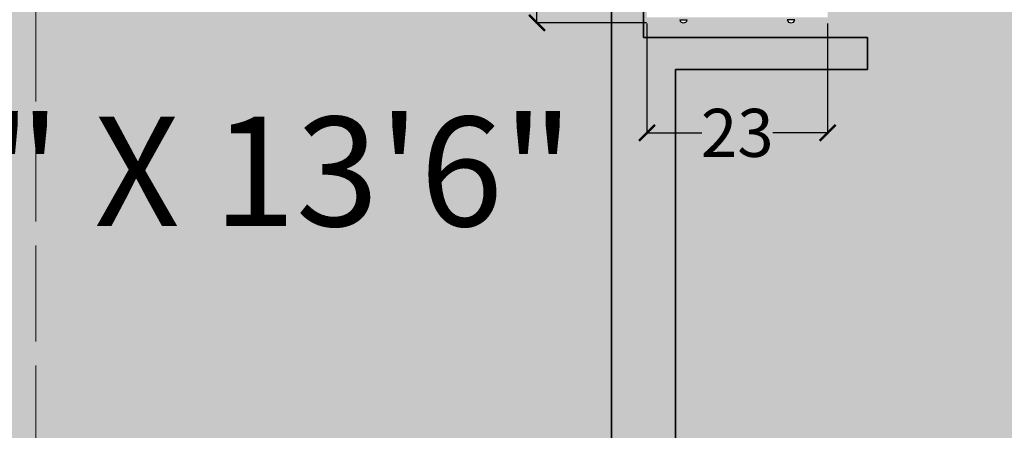
# Model space of a CAD drawing. Units: inches. Extents: x 1704 to 6393, y -157 to 1172.
# Tile 25 of 122: x 2275 to 2398, y 221 to 272. Entities that reach past the tile are written whole.
import ezdxf

# ---------------------------------------------------------------- set-up
doc = ezdxf.new("R2010")
doc.units = ezdxf.units.IN
doc.header["$MEASUREMENT"] = 0
doc.linetypes.add('ACAD_ISO02W100', pattern=[15, 12, -3])
for name, color, linetype, lineweight in [('A-ANNO-DIMS', 7, 'Continuous', 13), ('A-FURN', 8, 'Continuous', 18), ('A-WALL-OVHD', 8, 'ACAD_ISO02W100', 13), ('A-WALL-PATT', 7, 'Continuous', 13), ('estofado', 7, 'Continuous', 25), ('WALLS', 7, 'Continuous', 35)]:
    doc.layers.add(name, color=color, linetype=linetype, lineweight=lineweight)
doc.layers.add('A-FLOR-PATT', color=7, linetype='Continuous', lineweight=13, true_color=0xf2f2f2)
doc.layers.add('L-HRDS-PATT', color=9, linetype='Continuous', lineweight=13, true_color=0xc5c1ba)
doc.styles.get("Standard").update_dxf_attribs({"font": 'arial.ttf'})
doc.dimstyles.get("Standard").update_dxf_attribs({"dimtxt": 6, "dimasz": 2, "dimexe": 0.18, "dimexo": 0.0625, "dimgap": 0.09, "dimtad": 0, "dimtih": 1, "dimtoh": 1, "dimdec": 1, "dimzin": 0, "dimdsep": 46, "dimlunit": 3, "dimtxsty": 'Standard', "dimblk": 'ARCHTICK', "dimcen": 0.09, "dimadec": 0, "dimazin": 0, "dimtfac": 1, "dimtdec": 1, "dimtofl": 0, "dimtmove": 0, "dimatfit": 3, "dimfxl": 1, "dimtolj": 1, "dimtzin": 0, "dimarcsym": 0})

# ---------------------------------------------------------------- blocks, each defined once
blk = doc.blocks.new('Aparador Aido WV')
at = {"layer": 'estofado', "ltscale": 0.5}
for p, q in [((-0.9067, -0.0817), (-0.9067, -0.1006)), ((-0.9067, -0.3683), (-0.9067, -0.3494))]:
    blk.add_line(p, q, dxfattribs=at)
for centre in [(-0.904, -0.0911), (-0.904, -0.3589)]:
    blk.add_arc(centre, 0.0098, 105.9849, 254.0151, dxfattribs=at)
blk = doc.blocks.new('_ArchTick')
at = {"color": 0, "linetype": 'ByBlock', "const_width": 0.15}
blk.add_lwpolyline([(-0.5, -0.5), (0.5, 0.5)], dxfattribs=at)
blk = doc.blocks.new('*D68')
at = {"layer": 'A-ANNO-DIMS', "color": 0, "lineweight": -2, "transparency": 16777216}
for p, q in [((2353.71, 363.77), (2339.83, 363.77)), ((2340.01, 363.77), (2340.01, 321.11)), ((2340.01, 272.07), (2340.01, 314.72)), ((2353.71, 272.07), (2339.83, 272.07))]:
    blk.add_line(p, q, dxfattribs=at)
at = {"layer": 'Defpoints', "color": 0, "lineweight": -3, "transparency": 16777216}
for p in [(2340.01, 363.77), (2353.77, 363.77), (2353.77, 272.07)]:
    blk.add_point(p, dxfattribs=at)
at = {"layer": 'A-ANNO-DIMS', "color": 0, "lineweight": -2, "transparency": 16777216, "xscale": 2, "yscale": 2, "zscale": 2}
for p, rotation in [((2340.01, 363.77), 90), ((2340.01, 272.07), 270)]:
    blk.add_blockref('_ArchTick', p, dxfattribs=dict(at, rotation=rotation))
at = {"layer": 'A-ANNO-DIMS', "color": 0, "transparency": 16777216, "insert": (2340.01, 317.92), "char_height": 6, "attachment_point": 5}
blk.add_mtext('\\A1;SIDEBOARD 92', dxfattribs=at)
blk = doc.blocks.new('*D69')
at = {"layer": 'A-ANNO-DIMS', "color": 0, "lineweight": -2, "transparency": 16777216}
for p, q in [((2353.77, 272), (2353.77, 258.13)), ((2376.35, 272), (2376.35, 258.13)), ((2353.77, 258.31), (2360.62, 258.31)), ((2376.35, 258.31), (2369.5, 258.31))]:
    blk.add_line(p, q, dxfattribs=at)
at = {"layer": 'Defpoints', "color": 0, "lineweight": -3, "transparency": 16777216}
for p in [(2353.77, 272.07), (2376.35, 272.07), (2353.77, 258.31)]:
    blk.add_point(p, dxfattribs=at)
at = {"layer": 'A-ANNO-DIMS', "color": 0, "lineweight": -2, "transparency": 16777216, "xscale": 2, "yscale": 2, "zscale": 2, "rotation": 180}
blk.add_blockref('_ArchTick', (2353.77, 258.31), dxfattribs=at)
at = {"layer": 'A-ANNO-DIMS', "color": 0, "lineweight": -2, "transparency": 16777216, "xscale": 2, "yscale": 2, "zscale": 2}
blk.add_blockref('_ArchTick', (2376.35, 258.31), dxfattribs=at)
at = {"layer": 'A-ANNO-DIMS', "color": 0, "transparency": 16777216, "insert": (2365.06, 258.31), "char_height": 6, "attachment_point": 5}
blk.add_mtext('\\A1;23', dxfattribs=at)
blk = doc.blocks.new('*D93')
at = {"layer": 'A-ANNO-DIMS', "color": 0, "lineweight": -2, "transparency": 16777216}
for p, q in [((2605.29, 895.21), (1829.7, 895.21)), ((1829.88, 895.21), (1829.88, 495.87)), ((1829.88, 90.21), (1829.88, 489.56)), ((2605.29, 90.21), (1829.7, 90.21))]:
    blk.add_line(p, q, dxfattribs=at)
at = {"layer": 'Defpoints', "color": 0, "lineweight": -3, "transparency": 16777216}
for p in [(2605.35, 895.21), (1829.88, 90.21), (2605.35, 90.21)]:
    blk.add_point(p, dxfattribs=at)
at = {"layer": 'A-ANNO-DIMS', "color": 0, "lineweight": -2, "transparency": 16777216, "xscale": 2, "yscale": 2, "zscale": 2}
for p, rotation in [((1829.88, 895.21), 90), ((1829.88, 90.21), 270)]:
    blk.add_blockref('_ArchTick', p, dxfattribs=dict(at, rotation=rotation))
at = {"layer": 'A-ANNO-DIMS', "color": 0, "transparency": 16777216, "insert": (1829.88, 492.71), "char_height": 6, "attachment_point": 5}
blk.add_mtext('\\A1;805', dxfattribs=at)

msp = doc.modelspace()

# ---------------------------------------------------------------- hatches: boundary and pattern name
at = {"layer": 'A-FLOR-PATT', "transparency": 33554528}
h = msp.add_hatch(color=256, dxfattribs=at)
h.dxf.hatch_style = 1
h.paths.add_polyline_path([(2325.349, 863.213), (2325.349, 887.213), (2263.349, 887.213), (2167.349, 887.213), (2081.349, 887.213), (2081.349, 719.213), (2277.349, 719.213), (2277.349, 711.213), (2277.349, 372.213), (2349.349, 372.213), (2381.349, 372.213), (2381.349, 364.213), (2353.349, 364.213), (2353.349, 270.213), (2381.349, 270.213), (2381.349, 266.213), (2357.349, 266.213), (2357.349, 98.213), (2381.349, 98.213), (2385.181, 98.213), (2386.482, 98.213), (2424.215, 98.213), (2425.516, 98.213), (2429.349, 98.213), (2597.349, 98.213), (2597.349, 146.213), (2597.349, 218.213), (2597.349, 266.213), (2423.349, 266.213), (2423.349, 270.213), (2473.349, 270.213), (2473.349, 294.213), (2477.349, 294.213), (2477.349, 270.213), (2547.349, 270.213), (2547.349, 364.213), (2477.349, 364.213), (2477.349, 318.213), (2473.349, 318.213), (2473.349, 364.213), (2423.349, 364.213), (2423.349, 372.213), (2469.349, 372.213), (2469.349, 459.213), (2469.349, 538.213), (2350.349, 538.213), (2350.349, 565.713), (2358.349, 565.713), (2358.349, 545.213), (2420.349, 545.213), (2420.349, 610.213), (2358.349, 610.213), (2358.349, 589.713), (2350.349, 589.713), (2350.349, 615.213), (2425.349, 615.213), (2425.349, 607.213), (2425.349, 546.213), (2469.349, 546.213), (2514.349, 546.213), (2514.349, 607.213), (2449.349, 607.213), (2449.349, 615.213), (2451.738, 615.213), (2451.738, 659.213), (2427.738, 659.213), (2427.738, 665.213), (2367.738, 665.213), (2367.738, 667.213), (2367.738, 711.213), (2325.349, 711.213), (2325.349, 719.213), (2325.349, 755.213), (2325.349, 763.213)])
h.paths.add_polyline_path([(2233.858, 822.533, -0.187247), (2233.858, 809.14), (2231.697, 808.804, 0.0848928), (2233.131, 814.486), (2230.424, 814.486, -0.1042581), (2228.553, 808.313), (2217.751, 807.156, -0.2222222), (2217.751, 824.517), (2228.553, 823.359, -0.1042581), (2230.424, 817.186), (2233.131, 817.186, 0.0848928), (2231.697, 822.868)], flags=16)
h.paths.add_polyline_path([(2213.621, 833.197), (2213.621, 798.475), (2156.048, 798.475), (2156.048, 833.197)], flags=16)
h.paths.add_polyline_path([(2203.932, 848.099), (2205.089, 837.296, -0.2222222), (2187.728, 837.296), (2188.885, 848.099, -0.1042581), (2195.058, 849.969), (2195.058, 852.676, 0.0848928), (2189.377, 851.242), (2189.712, 853.404, -0.187247), (2203.105, 853.404), (2203.44, 851.242, 0.0848928), (2197.759, 852.676), (2197.759, 849.969, -0.1042581)], flags=16)
h.paths.add_polyline_path([(2181.941, 837.296, -0.2222222), (2164.58, 837.296), (2165.737, 848.099, -0.1042581), (2171.91, 849.969), (2171.91, 852.676, 0.0848928), (2166.229, 851.242), (2166.564, 853.404, -0.187247), (2179.957, 853.404), (2180.292, 851.242, 0.0848928), (2174.611, 852.676), (2174.611, 849.969, -0.1042581), (2180.784, 848.099)], flags=16)
h.paths.add_polyline_path([(2205.089, 794.376), (2203.932, 783.574, -0.1042581), (2197.759, 781.703), (2197.759, 778.996, 0.0848928), (2203.44, 780.43), (2203.105, 778.269, -0.187247), (2189.712, 778.269), (2189.377, 780.43, 0.0848928), (2195.058, 778.996), (2195.058, 781.703, -0.1042581), (2188.885, 783.574), (2187.728, 794.376, -0.2222222)], flags=16)
h.paths.add_polyline_path([(2181.941, 794.376), (2180.784, 783.574, -0.1042581), (2174.611, 781.703), (2174.611, 778.996, 0.0848928), (2180.292, 780.43), (2179.957, 778.269, -0.187247), (2166.564, 778.269), (2166.229, 780.43, 0.0848928), (2171.91, 778.996), (2171.91, 781.703, -0.1042581), (2165.737, 783.574), (2164.58, 794.376, -0.2222222)], flags=16)
h.paths.add_polyline_path([(2151.918, 807.156), (2141.116, 808.313, -0.1042581), (2139.245, 814.486), (2136.539, 814.486, 0.0848928), (2137.972, 808.804), (2135.811, 809.14, -0.187247), (2135.811, 822.533), (2137.972, 822.868, 0.0848928), (2136.539, 817.186), (2139.245, 817.186, -0.1042581), (2141.116, 823.359), (2151.918, 824.517, -0.2222222)], flags=16)
h.paths.add_polyline_path([(2357.868, 363.41), (2358.814, 363.41, 0.7537605)], flags=16)
h.paths.add_polyline_path([(2372.241, 363.117), (2372.248, 363.117), (2372.248, 363.343), (2371.302, 363.343), (2371.302, 363.139, -1.3603913)], flags=16)
h.paths.add_polyline_path([(2371.309, 272.716), (2371.302, 272.716), (2371.302, 272.49), (2372.248, 272.49), (2372.248, 272.693, -1.3603913)], flags=16)
h.paths.add_polyline_path([(2357.875, 272.716), (2357.868, 272.716), (2357.868, 272.49), (2358.814, 272.49), (2358.814, 272.693, -1.3603913)], flags=16)
h.paths.add_polyline_path([(2353.769, 363.074), (2376.347, 363.074), (2376.347, 272.759), (2353.769, 272.759)], flags=16)
h.paths.add_polyline_path([(2354.772, 362.07), (2375.344, 362.07), (2375.344, 273.762), (2354.772, 273.762)], flags=0)
h.paths.add_polyline_path([(2357.868, 363.343), (2358.814, 363.343), (2358.814, 363.117), (2357.868, 363.117)], flags=16)
h.paths.add_polyline_path([(2359.288, 359.184), (2359.288, 360.063), (2370.828, 360.063), (2370.828, 359.184), (2374.332, 359.184), (2374.332, 358.464), (2372.835, 358.464), (2372.835, 357.541), (2374.332, 357.541), (2374.332, 356.82), (2372.835, 356.82), (2372.835, 355.898), (2374.332, 355.898), (2374.332, 355.177), (2372.835, 355.177), (2372.835, 354.254), (2374.332, 354.254), (2374.332, 353.534), (2372.835, 353.534), (2372.835, 352.611), (2374.332, 352.611), (2374.332, 351.89), (2372.835, 351.89), (2372.835, 350.968), (2374.332, 350.968), (2374.332, 350.247), (2372.835, 350.247), (2372.835, 349.324), (2374.332, 349.324), (2374.332, 348.604), (2372.835, 348.604), (2372.835, 347.681), (2374.332, 347.681), (2374.332, 346.96), (2372.835, 346.96), (2372.835, 346.038), (2374.332, 346.038), (2374.332, 345.317), (2372.835, 345.317), (2372.835, 344.395), (2374.332, 344.395), (2374.332, 343.674), (2372.835, 343.674), (2372.835, 342.751), (2374.332, 342.751), (2374.332, 342.03), (2372.835, 342.03), (2372.835, 341.108), (2374.332, 341.108), (2374.332, 340.387), (2372.835, 340.387), (2372.835, 339.465), (2374.332, 339.465), (2374.332, 338.744), (2372.835, 338.744), (2372.835, 337.821), (2374.332, 337.821), (2374.332, 337.1), (2372.835, 337.1), (2372.835, 336.178), (2374.332, 336.178), (2374.332, 335.457), (2372.835, 335.457), (2372.835, 334.535), (2374.332, 334.535), (2374.332, 333.814), (2372.835, 333.814), (2372.835, 332.891), (2374.332, 332.891), (2374.332, 332.171), (2372.835, 332.171), (2372.835, 331.248), (2374.332, 331.248), (2374.332, 330.527), (2372.835, 330.527), (2372.835, 329.605), (2374.332, 329.605), (2374.332, 328.884), (2372.835, 328.884), (2372.835, 327.961), (2374.332, 327.961), (2374.332, 327.241), (2372.835, 327.241), (2372.835, 326.318), (2374.332, 326.318), (2374.332, 325.597), (2372.835, 325.597), (2372.835, 324.675), (2374.332, 324.675), (2374.332, 323.954), (2372.835, 323.954), (2372.835, 323.031), (2374.332, 323.031), (2374.332, 322.311), (2372.835, 322.311), (2372.835, 321.388), (2374.332, 321.388), (2374.332, 320.667), (2372.835, 320.667), (2372.835, 319.745), (2374.332, 319.745), (2374.332, 319.024), (2372.835, 319.024), (2372.835, 318.102), (2374.332, 318.102), (2374.332, 317.381), (2372.835, 317.381), (2372.835, 316.458), (2374.332, 316.458), (2374.332, 315.737), (2372.835, 315.737), (2372.835, 314.815), (2374.332, 314.815), (2374.332, 314.094), (2372.835, 314.094), (2372.835, 313.172), (2374.332, 313.172), (2374.332, 312.451), (2372.835, 312.451), (2372.835, 311.528), (2374.332, 311.528), (2374.332, 310.807), (2372.835, 310.807), (2372.835, 309.885), (2374.332, 309.885), (2374.332, 309.164), (2372.835, 309.164), (2372.835, 308.242), (2374.332, 308.242), (2374.332, 307.521), (2372.835, 307.521), (2372.835, 306.598), (2374.332, 306.598), (2374.332, 305.878), (2372.835, 305.878), (2372.835, 304.955), (2374.332, 304.955), (2374.332, 304.234), (2372.835, 304.234), (2372.835, 303.312), (2374.332, 303.312), (2374.332, 302.591), (2372.835, 302.591), (2372.835, 301.668), (2374.332, 301.668), (2374.332, 300.948), (2372.835, 300.948), (2372.835, 300.025), (2374.332, 300.025), (2374.332, 299.304), (2372.835, 299.304), (2372.835, 298.382), (2374.332, 298.382), (2374.332, 297.661), (2372.835, 297.661), (2372.835, 296.738), (2374.332, 296.738), (2374.332, 296.018), (2372.835, 296.018), (2372.835, 295.095), (2374.332, 295.095), (2374.332, 294.374), (2372.835, 294.374), (2372.835, 293.452), (2374.332, 293.452), (2374.332, 292.731), (2372.835, 292.731), (2372.835, 291.809), (2374.332, 291.809), (2374.332, 291.088), (2372.835, 291.088), (2372.835, 290.165), (2374.332, 290.165), (2374.332, 289.444), (2372.835, 289.444), (2372.835, 288.522), (2374.332, 288.522), (2374.332, 287.801), (2372.835, 287.801), (2372.835, 286.879), (2374.332, 286.879), (2374.332, 286.158), (2372.835, 286.158), (2372.835, 285.235), (2374.332, 285.235), (2374.332, 284.514), (2372.835, 284.514), (2372.835, 283.592), (2374.332, 283.592), (2374.332, 282.871), (2372.835, 282.871), (2372.835, 281.949), (2374.332, 281.949), (2374.332, 281.228), (2372.835, 281.228), (2372.835, 280.305), (2374.332, 280.305), (2374.332, 279.585), (2372.835, 279.585), (2372.835, 278.662), (2374.332, 278.662), (2374.332, 277.941), (2372.835, 277.941), (2372.835, 277.019), (2374.332, 277.019), (2374.332, 276.298), (2370.828, 276.298), (2370.828, 275.769), (2359.288, 275.769), (2359.288, 276.298), (2355.784, 276.298), (2355.784, 277.019), (2357.281, 277.019), (2357.281, 277.941), (2355.784, 277.941), (2355.784, 278.662), (2357.281, 278.662), (2357.281, 279.585), (2355.784, 279.585), (2355.784, 280.305), (2357.281, 280.305), (2357.281, 281.228), (2355.784, 281.228), (2355.784, 281.949), (2357.281, 281.949), (2357.281, 282.871), (2355.784, 282.871), (2355.784, 283.592), (2357.281, 283.592), (2357.281, 284.514), (2355.784, 284.514), (2355.784, 285.235), (2357.281, 285.235), (2357.281, 286.158), (2355.784, 286.158), (2355.784, 286.879), (2357.281, 286.879), (2357.281, 287.801), (2355.784, 287.801), (2355.784, 288.522), (2357.281, 288.522), (2357.281, 289.444), (2355.784, 289.444), (2355.784, 290.165), (2357.281, 290.165), (2357.281, 291.088), (2355.784, 291.088), (2355.784, 291.809), (2357.281, 291.809), (2357.281, 292.731), (2355.784, 292.731), (2355.784, 293.452), (2357.281, 293.452), (2357.281, 294.374), (2355.784, 294.374), (2355.784, 295.095), (2357.281, 295.095), (2357.281, 296.018), (2355.784, 296.018), (2355.784, 296.738), (2357.281, 296.738), (2357.281, 297.661), (2355.784, 297.661), (2355.784, 298.382), (2357.281, 298.382), (2357.281, 299.304), (2355.784, 299.304), (2355.784, 300.025), (2357.281, 300.025), (2357.281, 300.948), (2355.784, 300.948), (2355.784, 301.668), (2357.281, 301.668), (2357.281, 302.591), (2355.784, 302.591), (2355.784, 303.312), (2357.281, 303.312), (2357.281, 304.234), (2355.784, 304.234), (2355.784, 304.955), (2357.281, 304.955), (2357.281, 305.878), (2355.784, 305.878), (2355.784, 306.598), (2357.281, 306.598), (2357.281, 307.521), (2355.784, 307.521), (2355.784, 308.242), (2357.281, 308.242), (2357.281, 309.164), (2355.784, 309.164), (2355.784, 309.885), (2357.281, 309.885), (2357.281, 310.807), (2355.784, 310.807), (2355.784, 311.528), (2357.281, 311.528), (2357.281, 312.451), (2355.784, 312.451), (2355.784, 313.172), (2357.281, 313.172), (2357.281, 314.094), (2355.784, 314.094), (2355.784, 314.815), (2357.281, 314.815), (2357.281, 315.737), (2355.784, 315.737), (2355.784, 316.458), (2357.281, 316.458), (2357.281, 317.381), (2355.784, 317.381), (2355.784, 318.102), (2357.281, 318.102), (2357.281, 319.024), (2355.784, 319.024), (2355.784, 319.745), (2357.281, 319.745), (2357.281, 320.667), (2355.784, 320.667), (2355.784, 321.388), (2357.281, 321.388), (2357.281, 322.311), (2355.784, 322.311), (2355.784, 323.031), (2357.281, 323.031), (2357.281, 323.954), (2355.784, 323.954), (2355.784, 324.675), (2357.281, 324.675), (2357.281, 325.597), (2355.784, 325.597), (2355.784, 326.318), (2357.281, 326.318), (2357.281, 327.241), (2355.784, 327.241), (2355.784, 327.961), (2357.281, 327.961), (2357.281, 328.884), (2355.784, 328.884), (2355.784, 329.605), (2357.281, 329.605), (2357.281, 330.527), (2355.784, 330.527), (2355.784, 331.248), (2357.281, 331.248), (2357.281, 332.171), (2355.784, 332.171), (2355.784, 332.891), (2357.281, 332.891), (2357.281, 333.814), (2355.784, 333.814), (2355.784, 334.535), (2357.281, 334.535), (2357.281, 335.457), (2355.784, 335.457), (2355.784, 336.178), (2357.281, 336.178), (2357.281, 337.1), (2355.784, 337.1), (2355.784, 337.821), (2357.281, 337.821), (2357.281, 338.744), (2355.784, 338.744), (2355.784, 339.465), (2357.281, 339.465), (2357.281, 340.387), (2355.784, 340.387), (2355.784, 341.108), (2357.281, 341.108), (2357.281, 342.03), (2355.784, 342.03), (2355.784, 342.751), (2357.281, 342.751), (2357.281, 343.674), (2355.784, 343.674), (2355.784, 344.395), (2357.281, 344.395), (2357.281, 345.317), (2355.784, 345.317), (2355.784, 346.038), (2357.281, 346.038), (2357.281, 346.96), (2355.784, 346.96), (2355.784, 347.681), (2357.281, 347.681), (2357.281, 348.604), (2355.784, 348.604), (2355.784, 349.324), (2357.281, 349.324), (2357.281, 350.247), (2355.784, 350.247), (2355.784, 350.968), (2357.281, 350.968), (2357.281, 351.89), (2355.784, 351.89), (2355.784, 352.611), (2357.281, 352.611), (2357.281, 353.534), (2355.784, 353.534), (2355.784, 354.254), (2357.281, 354.254), (2357.281, 355.177), (2355.784, 355.177), (2355.784, 355.898), (2357.281, 355.898), (2357.281, 356.82), (2355.784, 356.82), (2355.784, 357.541), (2357.281, 357.541), (2357.281, 358.464), (2355.784, 358.464), (2355.784, 359.184)], flags=0)
h = msp.add_hatch(color=256, dxfattribs=at)
h.dxf.hatch_style = 1
h.paths.add_polyline_path([(2349.349, 372.213), (2277.349, 372.213), (2277.349, 364.213), (2349.349, 364.213)])
h.paths.add_polyline_path([(2277.349, 372.213), (2273.349, 372.213), (2273.349, 364.213), (2277.349, 364.213)])
h.paths.add_polyline_path([(2277.349, 364.213), (2273.349, 364.213), (2273.349, 202.213), (2277.349, 202.213)])
h.paths.add_polyline_path([(2277.349, 538.213), (2273.349, 538.213), (2273.349, 372.213), (2277.349, 372.213)])
h.paths.add_polyline_path([(2277.349, 629.213), (2273.349, 629.213), (2273.349, 545.213), (2277.349, 545.213)])
h.paths.add_polyline_path([(2277.349, 711.213), (2273.349, 711.213), (2273.349, 631.213), (2277.349, 631.213)])
h.paths.add_polyline_path([(2277.349, 631.213), (2273.349, 631.213), (2273.349, 629.213), (2277.349, 629.213)])
at = {"layer": 'A-WALL-PATT', "transparency": 33554643}
h = msp.add_hatch(color=256, dxfattribs=at)
h.dxf.hatch_style = 1
h.paths.add_polyline_path([(2167.349, 895.213), (2073.349, 895.213), (2073.349, 887.213), (2081.349, 887.213), (2167.349, 887.213)])
h.paths.add_polyline_path([(2465.349, 895.213), (2273.349, 895.213), (2273.349, 903.213), (2263.349, 903.213), (2263.349, 895.213), (2263.349, 887.213), (2325.349, 887.213), (2325.349, 863.213), (2333.349, 863.213), (2333.349, 887.213), (2465.349, 887.213)])
h.paths.add_polyline_path([(2533.349, 895.213), (2513.349, 895.213), (2513.349, 887.213), (2513.349, 861.213), (2517.349, 861.213), (2517.349, 887.213), (2533.349, 887.213)])
h.paths.add_polyline_path([(2605.349, 895.213), (2581.349, 895.213), (2581.349, 887.213), (2597.349, 887.213), (2597.349, 854.213), (2605.349, 854.213)])
h.paths.add_polyline_path([(2605.349, 752.213), (2629.349, 752.213), (2629.349, 716.213), (2605.349, 716.213), (2605.349, 712.213), (2719.349, 712.213), (2719.349, 716.213), (2631.349, 716.213), (2631.349, 754.213), (2605.349, 754.213), (2605.349, 794.213), (2597.349, 794.213), (2597.349, 787.213), (2517.349, 787.213), (2517.349, 813.213), (2513.349, 813.213), (2513.349, 783.213), (2517.349, 783.213), (2597.349, 783.213), (2597.349, 719.213), (2517.349, 719.213), (2517.349, 753.213), (2513.349, 753.213), (2513.349, 719.213), (2365.349, 719.213), (2365.349, 763.213), (2325.349, 763.213), (2325.349, 755.213), (2357.349, 755.213), (2357.349, 719.213), (2325.349, 719.213), (2325.349, 711.213), (2547.349, 711.213), (2547.349, 615.213), (2449.349, 615.213), (2449.349, 607.213), (2514.349, 607.213), (2514.349, 546.213), (2439.349, 546.213), (2425.349, 546.213), (2425.349, 607.213), (2425.349, 615.213), (2350.349, 615.213), (2350.349, 589.713), (2358.349, 589.713), (2358.349, 610.213), (2420.349, 610.213), (2420.349, 545.213), (2358.349, 545.213), (2358.349, 565.713), (2350.349, 565.713), (2350.349, 538.213), (2469.349, 538.213), (2469.349, 459.213), (2469.349, 372.213), (2423.349, 372.213), (2423.349, 364.213), (2473.349, 364.213), (2473.349, 318.213), (2477.349, 318.213), (2477.349, 364.213), (2547.349, 364.213), (2547.349, 352.213), (2549.349, 352.213), (2549.349, 364.213), (2597.349, 364.213), (2597.349, 328.213), (2549.349, 328.213), (2547.349, 328.213), (2547.349, 326.213), (2549.349, 326.213), (2597.349, 326.213), (2605.349, 326.213), (2605.349, 377.057), (2597.349, 377.057), (2597.349, 372.213), (2477.349, 372.213), (2477.349, 451.213), (2597.349, 451.213), (2605.349, 451.213), (2605.349, 459.213), (2597.349, 459.213), (2477.349, 459.213), (2477.349, 538.213), (2597.349, 538.213), (2597.349, 495.213), (2605.349, 495.213), (2605.349, 512.213), (2631.349, 512.213), (2631.349, 568.213), (2605.349, 568.213), (2605.349, 577.213), (2597.349, 577.213), (2597.349, 542.213), (2518.349, 542.213), (2518.349, 607.213), (2532.349, 607.213), (2605.349, 607.213), (2605.349, 615.213), (2597.349, 615.213), (2551.349, 615.213), (2551.349, 711.213), (2597.349, 711.213), (2597.349, 645.213), (2605.349, 645.213), (2605.349, 712.213), (2605.349, 716.213)])
h.paths.add_polyline_path([(2605.349, 566.213), (2629.349, 566.213), (2629.349, 514.213), (2605.349, 514.213)], flags=16)
h.paths.add_polyline_path([(2381.349, 372.213), (2349.349, 372.213), (2349.349, 202.213), (2337.349, 202.213), (2337.349, 194.213), (2349.349, 194.213), (2349.349, 90.213), (2349.349, 72.213), (2357.349, 72.213), (2357.349, 90.213), (2381.349, 90.213), (2381.349, 98.213), (2357.349, 98.213), (2357.349, 266.213), (2381.349, 266.213), (2381.349, 270.213), (2353.349, 270.213), (2353.349, 364.213), (2381.349, 364.213)])
h.paths.add_polyline_path([(2605.349, 302.213), (2597.349, 302.213), (2597.349, 270.213), (2477.349, 270.213), (2477.349, 294.213), (2473.349, 294.213), (2473.349, 270.213), (2423.349, 270.213), (2423.349, 266.213), (2597.349, 266.213), (2597.349, 218.213), (2605.349, 218.213)])
h.paths.add_polyline_path([(2605.349, 146.213), (2597.349, 146.213), (2597.349, 98.213), (2429.349, 98.213), (2429.349, 90.213), (2597.349, 90.213), (2597.349, 72.213), (2605.349, 72.213), (2605.349, 90.213)])
h.paths.add_polyline_path([(2225.349, 202.213), (2049.349, 202.213), (2049.349, 194.213), (2225.349, 194.213)])
h.paths.add_polyline_path([(2289.349, 202.213), (2277.349, 202.213), (2273.349, 202.213), (2269.516, 202.213), (2269.516, 194.213), (2273.349, 194.213), (2277.349, 194.213), (2289.349, 194.213)])
h.paths.add_polyline_path([(2273.349, 372.213), (2029.19, 372.213), (2029.19, 364.213), (2273.349, 364.213)])
h.paths.add_polyline_path([(2277.349, 545.213), (2213.349, 545.213), (2213.349, 573.213), (2205.349, 573.213), (2177.349, 573.213), (2177.349, 545.213), (2073.349, 545.213), (2073.349, 538.213), (2081.349, 538.213), (2277.349, 538.213)])
h.paths.add_polyline_path([(2181.349, 545.213), (2181.349, 569.213), (2205.349, 569.213), (2205.349, 545.213)], flags=16)
h.paths.add_polyline_path([(2277.349, 719.213), (2081.349, 719.213), (2073.349, 719.213), (2073.349, 711.213), (2154.575, 711.213), (2205.349, 711.213), (2205.349, 687.213), (2205.349, 629.213), (2213.349, 629.213), (2273.349, 629.213), (2273.349, 631.213), (2207.349, 631.213), (2207.349, 707.213), (2231.349, 707.213), (2231.349, 709.213), (2207.349, 709.213), (2207.349, 711.213), (2277.349, 711.213)])
at = {"layer": 'L-HRDS-PATT', "transparency": 33554539}
h = msp.add_hatch(color=256, dxfattribs=at)
h.dxf.hatch_style = 1
h.paths.add_polyline_path([(2651.217, 368.213), (2605.349, 368.213), (2605.349, 218.213), (2605.349, 212.464), (2605.349, 210.513), (2605.349, 153.913), (2605.349, 151.962), (2605.349, 146.213), (2605.349, 90.213), (2605.349, 72.213), (2601.349, 72.213), (2600.88, 50.634), (2719.349, 50.634), (2719.349, 72.213), (2711.349, 72.213), (2663.217, 72.213), (2651.217, 72.213)])
h.paths.add_polyline_path([(2711.349, 48.634), (2600.88, 48.634), (2576.88, 48.634), (2576.88, 17.658), (2711.349, 17.658)])
h.paths.add_polyline_path([(2601.349, 72.213), (2597.349, 72.213), (2597.349, 90.213), (2429.349, 90.213), (2425.516, 90.213), (2424.215, 90.213), (2386.482, 90.213), (2385.181, 90.213), (2381.349, 90.213), (2357.349, 90.213), (2357.349, 72.213), (2349.349, 72.213), (2349.349, 90.213), (2349.349, 134.213), (2277.349, 134.213), (2277.349, 50.634), (2566.88, 50.634), (2600.88, 50.634)])
h.paths.add_polyline_path([(2349.349, 146.213), (2277.349, 146.213), (2277.349, 134.213), (2349.349, 134.213)])
h.paths.add_polyline_path([(2349.349, 158.213), (2277.349, 158.213), (2277.349, 146.213), (2349.349, 146.213)])
h.paths.add_polyline_path([(2349.349, 170.213), (2277.349, 170.213), (2277.349, 158.213), (2349.349, 158.213)])
h.paths.add_polyline_path([(2349.349, 194.213), (2337.349, 194.213), (2337.349, 202.213), (2349.349, 202.213), (2349.349, 364.213), (2277.349, 364.213), (2277.349, 202.213), (2289.349, 202.213), (2289.349, 194.213), (2277.349, 194.213), (2277.349, 170.213), (2349.349, 170.213)])

# ---------------------------------------------------------------- linework, layer by layer
at = {"layer": 'A-WALL-OVHD'}
msp.add_line((2277.349, 202.213), (2277.349, 711.213), dxfattribs=at)
at = {"layer": 'WALLS'}
for p, q in [((2349.349, 202.213), (2349.349, 372.213)), ((2353.349, 270.213), (2353.349, 364.213)), ((2381.349, 270.213), (2353.349, 270.213)), ((2381.349, 266.213), (2381.349, 270.213)), ((2357.349, 98.213), (2357.349, 266.213)), ((2381.349, 266.213), (2357.349, 266.213))]:
    msp.add_line(p, q, dxfattribs=at)

# ---------------------------------------------------------------- block references
at = {"layer": 'A-FURN', "xscale": 50.174952135231, "yscale": 50.174952135231, "zscale": 50.174952135231, "rotation": 90}
msp.add_blockref('Aparador Aido WV', (2353.769, 317.916), dxfattribs=at)

# ---------------------------------------------------------------- texts
at = {"layer": 'A-ANNO-DIMS'}
msp.add_text('6\'0" X 13\'6"', height=13.6672, dxfattribs=at).set_placement((2245.77, 246.646))

# ---------------------------------------------------------------- dimensions: what is measured, and where the dimension line sits
for base, p1, p2, angle, picture, middle in [((1829.878, 90.213), (2605.349, 895.213), (2605.349, 90.213), 90, '*D93', (1829.878, 492.713)), ((2353.769, 258.311), (2376.347, 272.066), (2353.769, 272.066), 180, '*D69', (2365.058, 258.311))]:
    dim = msp.add_linear_dim(base=base, p1=p1, p2=p2, angle=angle, dimstyle='Standard', override={"dimdec": 0, "dimlfac": 1, "dimrnd": 0, "dimzin": 0, "dimdsep": 46, "dimlunit": 2}, dxfattribs=at)
    dim.commit()
    dim.dimension.update_dxf_attribs({"geometry": picture, "text_midpoint": middle})
dim = msp.add_linear_dim(base=(2340.014, 363.767), p1=(2353.769, 272.066), p2=(2353.769, 363.767), angle=90, text='SIDEBOARD <>', dimstyle='Standard', override={"dimdec": 0, "dimlfac": 1, "dimrnd": 0, "dimzin": 0, "dimdsep": 46, "dimlunit": 2}, dxfattribs=at)
dim.commit()
dim.dimension.update_dxf_attribs({"geometry": '*D68', "text_midpoint": (2340.014, 317.916)})

doc.saveas('drawing.dxf')
